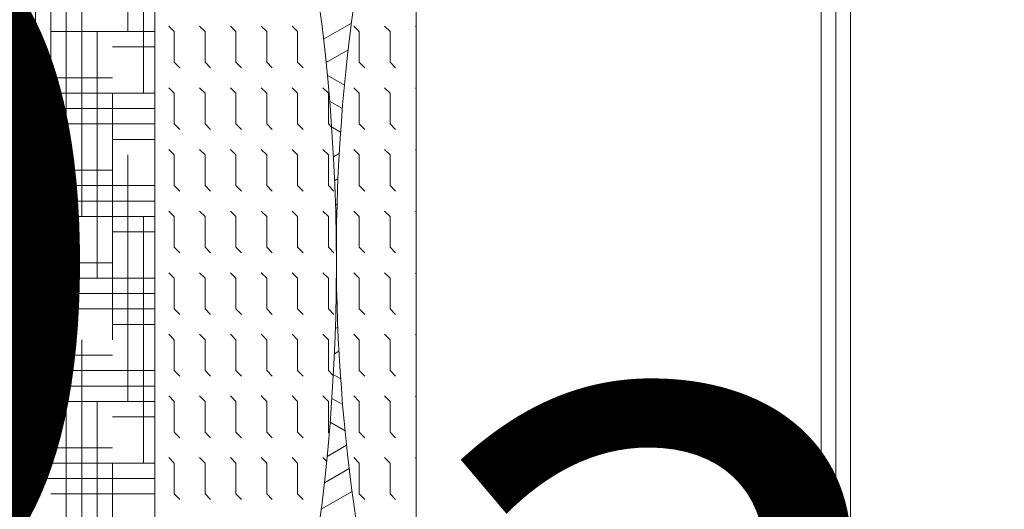
# Model space of a CAD drawing. Units: inches. Extents: x -90 to 536, y -553 to 299.
# Tile 6 of 27: x 96 to 122, y -375 to -362. Entities that reach past the tile are written whole.
import ezdxf

# ---------------------------------------------------------------- set-up
doc = ezdxf.new("R2010")
doc.units = ezdxf.units.IN
doc.layers.add('A-ANNO-DIMS', color=2, linetype='Continuous', lineweight=18)
doc.layers.add('Furniture', color=2, linetype='Continuous', lineweight=18)
doc.styles.get("Standard").update_dxf_attribs({"font": 'arial.ttf'})
doc.dimstyles.get("Standard").update_dxf_attribs({"dimtxt": 18, "dimasz": 12, "dimexe": 0.18, "dimexo": 0.0625, "dimgap": 0.09, "dimtad": 0, "dimtih": 1, "dimtoh": 1, "dimdec": 0, "dimzin": 0, "dimdsep": 46, "dimlunit": 3, "dimtxsty": 'Standard', "dimcen": 0.09, "dimadec": 0, "dimazin": 0, "dimtfac": 1, "dimtdec": 0, "dimtofl": 0, "dimtmove": 0, "dimatfit": 3, "dimfxl": 1, "dimtolj": 1, "dimtzin": 0, "dimarcsym": 0})

# ---------------------------------------------------------------- blocks, each defined once
blk = doc.blocks.new('A$C62731D1C')
for p, q in [((0.10613, 0.66415, 0.68571), (1.46095, 0.66415, 0.68571)), ((0.10613, 0.65215, 0.68571), (1.46095, 0.65215, 0.68571)), ((0.10613, 0.64015, 0.68571), (1.46095, 0.64015, 0.68571)), ((1.39167, 0.31204, 0.68571), (0.17247, 0.31204, 0.68571)), ((0.57908, 0.31135, 0.68571), (0.57977, 0.31204, 0.68571)), ((0.62908, 0.31135, 0.68571), (0.62977, 0.31204, 0.68571)), ((0.67908, 0.31135, 0.68571), (0.67977, 0.31204, 0.68571)), ((0.72908, 0.31135, 0.68571), (0.72977, 0.31204, 0.68571)), ((0.77908, 0.31135, 0.68571), (0.77977, 0.31204, 0.68571)), ((0.82908, 0.31135, 0.68571), (0.82977, 0.31204, 0.68571)), ((0.87908, 0.31135, 0.68571), (0.87977, 0.31204, 0.68571)), ((0.92908, 0.31135, 0.68571), (0.92977, 0.31204, 0.68571)), ((0.57908, 0.28635, 0.68571), (0.5835, 0.29077, 0.68571)), ((0.5835, 0.29077, 0.68571), (0.6085, 0.29077, 0.68571)), ((0.6085, 0.29077, 0.68571), (0.61292, 0.29519, 0.68571)), ((0.62908, 0.28635, 0.68571), (0.6335, 0.29077, 0.68571)), ((0.6335, 0.29077, 0.68571), (0.6585, 0.29077, 0.68571)), ((0.6585, 0.29077, 0.68571), (0.66292, 0.29519, 0.68571)), ((0.67908, 0.28635, 0.68571), (0.6835, 0.29077, 0.68571)), ((0.6835, 0.29077, 0.68571), (0.7085, 0.29077, 0.68571)), ((0.7085, 0.29077, 0.68571), (0.71292, 0.29519, 0.68571)), ((0.72908, 0.28635, 0.68571), (0.7335, 0.29077, 0.68571)), ((0.7335, 0.29077, 0.68571), (0.7585, 0.29077, 0.68571)), ((0.7585, 0.29077, 0.68571), (0.76292, 0.29519, 0.68571)), ((0.77908, 0.28635, 0.68571), (0.7835, 0.29077, 0.68571)), ((0.7835, 0.29077, 0.68571), (0.8085, 0.29077, 0.68571)), ((0.8085, 0.29077, 0.68571), (0.81292, 0.29519, 0.68571)), ((0.82908, 0.28635, 0.68571), (0.8335, 0.29077, 0.68571)), ((0.8335, 0.29077, 0.68571), (0.8585, 0.29077, 0.68571)), ((0.8585, 0.29077, 0.68571), (0.86292, 0.29519, 0.68571)), ((0.87908, 0.28635, 0.68571), (0.8835, 0.29077, 0.68571)), ((0.8835, 0.29077, 0.68571), (0.9085, 0.29077, 0.68571)), ((0.9085, 0.29077, 0.68571), (0.91292, 0.29519, 0.68571)), ((0.92908, 0.28635, 0.68571), (0.9335, 0.29077, 0.68571)), ((0.9335, 0.29077, 0.68571), (0.9585, 0.29077, 0.68571)), ((0.9585, 0.29077, 0.68571), (0.96292, 0.29519, 0.68571)), ((0.57908, 0.26135, 0.68571), (0.5835, 0.26577, 0.68571)), ((0.5835, 0.26577, 0.68571), (0.6085, 0.26577, 0.68571)), ((0.6085, 0.26577, 0.68571), (0.61292, 0.27019, 0.68571)), ((0.62908, 0.26135, 0.68571), (0.6335, 0.26577, 0.68571)), ((0.6335, 0.26577, 0.68571), (0.6585, 0.26577, 0.68571)), ((0.6585, 0.26577, 0.68571), (0.66292, 0.27019, 0.68571)), ((0.67908, 0.26135, 0.68571), (0.6835, 0.26577, 0.68571)), ((0.6835, 0.26577, 0.68571), (0.7085, 0.26577, 0.68571)), ((0.7085, 0.26577, 0.68571), (0.71292, 0.27019, 0.68571)), ((0.72908, 0.26135, 0.68571), (0.7335, 0.26577, 0.68571)), ((0.7335, 0.26577, 0.68571), (0.7585, 0.26577, 0.68571)), ((0.7585, 0.26577, 0.68571), (0.76292, 0.27019, 0.68571)), ((0.77908, 0.26135, 0.68571), (0.7835, 0.26577, 0.68571)), ((0.7835, 0.26577, 0.68571), (0.8085, 0.26577, 0.68571)), ((0.8085, 0.26577, 0.68571), (0.81292, 0.27019, 0.68571)), ((0.82908, 0.26135, 0.68571), (0.8335, 0.26577, 0.68571)), ((0.8335, 0.26577, 0.68571), (0.8585, 0.26577, 0.68571)), ((0.8585, 0.26577, 0.68571), (0.86292, 0.27019, 0.68571)), ((0.87908, 0.26135, 0.68571), (0.8835, 0.26577, 0.68571)), ((0.8835, 0.26577, 0.68571), (0.9085, 0.26577, 0.68571)), ((0.9085, 0.26577, 0.68571), (0.91292, 0.27019, 0.68571)), ((0.92908, 0.26135, 0.68571), (0.9335, 0.26577, 0.68571)), ((0.9335, 0.26577, 0.68571), (0.9585, 0.26577, 0.68571)), ((0.9585, 0.26577, 0.68571), (0.96292, 0.27019, 0.68571)), ((0.57677, 0.25948, 0.68571), (0.58983, 0.23685, 0.68571)), ((0.60866, 0.23889, 0.68571), (0.5983, 0.25682, 0.68571)), ((0.92819, 0.23969, 0.68571), (0.91906, 0.2555, 0.68571)), ((0.93782, 0.25765, 0.68571), (0.94947, 0.23748, 0.68571)), ((0.97092, 0.23496, 0.68571), (0.95645, 0.26002, 0.68571)), ((0.62695, 0.25378, 0.68571), (0.61894, 0.2399, 0.68571)), ((0.64002, 0.24179, 0.68571), (0.64597, 0.25209, 0.68571)), ((0.66513, 0.25064, 0.68571), (0.66094, 0.24338, 0.68571)), ((0.6852, 0.24488, 0.68571), (0.6825, 0.24954, 0.68571)), ((0.70309, 0.24852, 0.68571), (0.70465, 0.24582, 0.68571)), ((0.72425, 0.24652, 0.68571), (0.72351, 0.24779, 0.68571)), ((0.80401, 0.24693, 0.68571), (0.80355, 0.24773, 0.68571)), ((0.82316, 0.2484, 0.68571), (0.82431, 0.24641, 0.68571)), ((0.84477, 0.24562, 0.68571), (0.84263, 0.24932, 0.68571)), ((0.86518, 0.25072, 0.68571), (0.86174, 0.24476, 0.68571)), ((0.88105, 0.24357, 0.68571), (0.88611, 0.25234, 0.68571)), ((0.90723, 0.25428, 0.68571), (0.90024, 0.24216, 0.68571)), ((0.62908, 0.23635, 0.68571), (0.6335, 0.24077, 0.68571)), ((0.6335, 0.24077, 0.68571), (0.6585, 0.24077, 0.68571)), ((0.6585, 0.24077, 0.68571), (0.66112, 0.24339, 0.68571)), ((0.67908, 0.23635, 0.68571), (0.6835, 0.24077, 0.68571)), ((0.6835, 0.24077, 0.68571), (0.7085, 0.24077, 0.68571)), ((0.7085, 0.24077, 0.68571), (0.71292, 0.24519, 0.68571)), ((0.72908, 0.23635, 0.68571), (0.7335, 0.24077, 0.68571)), ((0.7335, 0.24077, 0.68571), (0.7585, 0.24077, 0.68571)), ((0.74324, 0.24737, 0.68571), (0.74302, 0.24697, 0.68571)), ((0.7585, 0.24077, 0.68571), (0.76292, 0.24519, 0.68571)), ((0.77908, 0.23635, 0.68571), (0.7835, 0.24077, 0.68571)), ((0.78322, 0.24733, 0.68571), (0.78315, 0.24721, 0.68571)), ((0.7835, 0.24077, 0.68571), (0.8085, 0.24077, 0.68571)), ((0.8085, 0.24077, 0.68571), (0.81292, 0.24519, 0.68571)), ((0.82908, 0.23635, 0.68571), (0.8335, 0.24077, 0.68571)), ((0.8335, 0.24077, 0.68571), (0.8585, 0.24077, 0.68571)), ((0.8585, 0.24077, 0.68571), (0.86246, 0.24472, 0.68571)), ((0.87908, 0.23635, 0.68571), (0.8835, 0.24077, 0.68571)), ((0.8835, 0.24077, 0.68571), (0.9085, 0.24077, 0.68571)), ((0.9085, 0.24077, 0.68571), (0.90916, 0.24143, 0.68571)), ((0.92908, 0.23635, 0.68571), (0.93204, 0.23931, 0.68571)), ((0.57908, 0.21135, 0.68571), (0.5835, 0.21577, 0.68571)), ((0.5835, 0.21577, 0.68571), (0.6085, 0.21577, 0.68571)), ((0.6085, 0.21577, 0.68571), (0.61292, 0.22019, 0.68571)), ((0.62908, 0.21135, 0.68571), (0.6335, 0.21577, 0.68571)), ((0.6335, 0.21577, 0.68571), (0.6585, 0.21577, 0.68571)), ((0.6585, 0.21577, 0.68571), (0.66292, 0.22019, 0.68571)), ((0.67908, 0.21135, 0.68571), (0.6835, 0.21577, 0.68571)), ((0.6835, 0.21577, 0.68571), (0.7085, 0.21577, 0.68571)), ((0.7085, 0.21577, 0.68571), (0.71292, 0.22019, 0.68571)), ((0.72908, 0.21135, 0.68571), (0.7335, 0.21577, 0.68571)), ((0.7335, 0.21577, 0.68571), (0.7585, 0.21577, 0.68571)), ((0.7585, 0.21577, 0.68571), (0.76292, 0.22019, 0.68571)), ((0.77908, 0.21135, 0.68571), (0.7835, 0.21577, 0.68571)), ((0.7835, 0.21577, 0.68571), (0.8085, 0.21577, 0.68571)), ((0.8085, 0.21577, 0.68571), (0.81292, 0.22019, 0.68571)), ((0.82908, 0.21135, 0.68571), (0.8335, 0.21577, 0.68571)), ((0.8335, 0.21577, 0.68571), (0.8585, 0.21577, 0.68571)), ((0.8585, 0.21577, 0.68571), (0.86292, 0.22019, 0.68571)), ((0.87908, 0.21135, 0.68571), (0.8835, 0.21577, 0.68571)), ((0.8835, 0.21577, 0.68571), (0.9085, 0.21577, 0.68571)), ((0.9085, 0.21577, 0.68571), (0.91292, 0.22019, 0.68571)), ((0.92908, 0.21135, 0.68571), (0.9335, 0.21577, 0.68571)), ((0.9335, 0.21577, 0.68571), (0.9585, 0.21577, 0.68571)), ((0.9585, 0.21577, 0.68571), (0.96292, 0.22019, 0.68571)), ((0.6085, 0.19077, 0.68571), (0.61292, 0.19519, 0.68571)), ((0.6585, 0.19077, 0.68571), (0.66292, 0.19519, 0.68571)), ((0.7085, 0.19077, 0.68571), (0.71292, 0.19519, 0.68571)), ((0.7585, 0.19077, 0.68571), (0.76292, 0.19519, 0.68571)), ((0.8085, 0.19077, 0.68571), (0.81292, 0.19519, 0.68571)), ((0.8585, 0.19077, 0.68571), (0.86292, 0.19519, 0.68571)), ((0.9085, 0.19077, 0.68571), (0.91292, 0.19519, 0.68571)), ((0.9585, 0.19077, 0.68571), (0.96292, 0.19519, 0.68571)), ((0.57908, 0.18635, 0.68571), (0.5835, 0.19077, 0.68571)), ((0.5835, 0.19077, 0.68571), (0.6085, 0.19077, 0.68571)), ((0.62908, 0.18635, 0.68571), (0.6335, 0.19077, 0.68571)), ((0.6335, 0.19077, 0.68571), (0.6585, 0.19077, 0.68571)), ((0.67908, 0.18635, 0.68571), (0.6835, 0.19077, 0.68571)), ((0.6835, 0.19077, 0.68571), (0.7085, 0.19077, 0.68571)), ((0.72908, 0.18635, 0.68571), (0.7335, 0.19077, 0.68571)), ((0.7335, 0.19077, 0.68571), (0.7585, 0.19077, 0.68571)), ((0.77908, 0.18635, 0.68571), (0.7835, 0.19077, 0.68571)), ((0.7835, 0.19077, 0.68571), (0.8085, 0.19077, 0.68571)), ((0.82908, 0.18635, 0.68571), (0.8335, 0.19077, 0.68571)), ((0.8335, 0.19077, 0.68571), (0.8585, 0.19077, 0.68571)), ((0.87908, 0.18635, 0.68571), (0.8835, 0.19077, 0.68571)), ((0.8835, 0.19077, 0.68571), (0.9085, 0.19077, 0.68571)), ((0.92908, 0.18635, 0.68571), (0.9335, 0.19077, 0.68571)), ((0.9335, 0.19077, 0.68571), (0.9585, 0.19077, 0.68571)), ((0.6085, 0.16577, 0.68571), (0.61292, 0.17019, 0.68571)), ((0.6585, 0.16577, 0.68571), (0.66292, 0.17019, 0.68571)), ((0.7085, 0.16577, 0.68571), (0.71292, 0.17019, 0.68571)), ((0.7585, 0.16577, 0.68571), (0.76292, 0.17019, 0.68571)), ((0.8085, 0.16577, 0.68571), (0.81292, 0.17019, 0.68571)), ((0.8585, 0.16577, 0.68571), (0.86292, 0.17019, 0.68571)), ((0.9085, 0.16577, 0.68571), (0.91292, 0.17019, 0.68571)), ((0.9585, 0.16577, 0.68571), (0.96292, 0.17019, 0.68571)), ((0.57908, 0.16135, 0.68571), (0.5835, 0.16577, 0.68571)), ((0.5835, 0.16577, 0.68571), (0.6085, 0.16577, 0.68571)), ((0.62908, 0.16135, 0.68571), (0.6335, 0.16577, 0.68571)), ((0.6335, 0.16577, 0.68571), (0.6585, 0.16577, 0.68571)), ((0.67908, 0.16135, 0.68571), (0.6835, 0.16577, 0.68571)), ((0.6835, 0.16577, 0.68571), (0.7085, 0.16577, 0.68571)), ((0.72908, 0.16135, 0.68571), (0.7335, 0.16577, 0.68571)), ((0.7335, 0.16577, 0.68571), (0.7585, 0.16577, 0.68571)), ((0.77908, 0.16135, 0.68571), (0.7835, 0.16577, 0.68571)), ((0.7835, 0.16577, 0.68571), (0.8085, 0.16577, 0.68571)), ((0.82908, 0.16135, 0.68571), (0.8335, 0.16577, 0.68571)), ((0.8335, 0.16577, 0.68571), (0.8585, 0.16577, 0.68571)), ((0.87908, 0.16135, 0.68571), (0.8835, 0.16577, 0.68571)), ((0.8835, 0.16577, 0.68571), (0.9085, 0.16577, 0.68571)), ((0.92908, 0.16135, 0.68571), (0.9335, 0.16577, 0.68571)), ((0.9335, 0.16577, 0.68571), (0.9585, 0.16577, 0.68571)), ((0.6085, 0.14077, 0.68571), (0.61292, 0.14519, 0.68571)), ((0.6585, 0.14077, 0.68571), (0.66292, 0.14519, 0.68571)), ((0.7085, 0.14077, 0.68571), (0.71292, 0.14519, 0.68571)), ((0.7585, 0.14077, 0.68571), (0.76292, 0.14519, 0.68571)), ((0.8085, 0.14077, 0.68571), (0.81292, 0.14519, 0.68571)), ((0.8585, 0.14077, 0.68571), (0.86292, 0.14519, 0.68571)), ((0.9085, 0.14077, 0.68571), (0.91292, 0.14519, 0.68571)), ((0.9585, 0.14077, 0.68571), (0.96292, 0.14519, 0.68571)), ((0.57908, 0.13635, 0.68571), (0.5835, 0.14077, 0.68571)), ((0.5835, 0.14077, 0.68571), (0.6085, 0.14077, 0.68571)), ((0.62908, 0.13635, 0.68571), (0.6335, 0.14077, 0.68571)), ((0.6335, 0.14077, 0.68571), (0.6585, 0.14077, 0.68571)), ((0.67908, 0.13635, 0.68571), (0.6835, 0.14077, 0.68571)), ((0.6835, 0.14077, 0.68571), (0.7085, 0.14077, 0.68571)), ((0.72908, 0.13635, 0.68571), (0.7335, 0.14077, 0.68571)), ((0.7335, 0.14077, 0.68571), (0.7585, 0.14077, 0.68571)), ((0.77908, 0.13635, 0.68571), (0.7835, 0.14077, 0.68571)), ((0.7835, 0.14077, 0.68571), (0.8085, 0.14077, 0.68571)), ((0.82908, 0.13635, 0.68571), (0.8335, 0.14077, 0.68571)), ((0.8335, 0.14077, 0.68571), (0.8585, 0.14077, 0.68571)), ((0.87908, 0.13635, 0.68571), (0.8835, 0.14077, 0.68571)), ((0.8835, 0.14077, 0.68571), (0.9085, 0.14077, 0.68571)), ((0.92908, 0.13635, 0.68571), (0.9335, 0.14077, 0.68571)), ((0.9335, 0.14077, 0.68571), (0.9585, 0.14077, 0.68571)), ((0.6085, 0.11577, 0.68571), (0.61292, 0.12019, 0.68571)), ((0.6585, 0.11577, 0.68571), (0.66292, 0.12019, 0.68571)), ((0.7085, 0.11577, 0.68571), (0.71292, 0.12019, 0.68571)), ((0.7585, 0.11577, 0.68571), (0.76292, 0.12019, 0.68571)), ((0.8085, 0.11577, 0.68571), (0.81292, 0.12019, 0.68571)), ((0.8585, 0.11577, 0.68571), (0.86292, 0.12019, 0.68571)), ((0.9085, 0.11577, 0.68571), (0.91292, 0.12019, 0.68571)), ((0.9585, 0.11577, 0.68571), (0.96292, 0.12019, 0.68571)), ((0.57908, 0.11135, 0.68571), (0.5835, 0.11577, 0.68571)), ((0.5835, 0.11577, 0.68571), (0.6085, 0.11577, 0.68571)), ((0.62908, 0.11135, 0.68571), (0.6335, 0.11577, 0.68571)), ((0.6335, 0.11577, 0.68571), (0.6585, 0.11577, 0.68571)), ((0.67908, 0.11135, 0.68571), (0.6835, 0.11577, 0.68571)), ((0.6835, 0.11577, 0.68571), (0.7085, 0.11577, 0.68571)), ((0.72908, 0.11135, 0.68571), (0.7335, 0.11577, 0.68571)), ((0.7335, 0.11577, 0.68571), (0.7585, 0.11577, 0.68571)), ((0.77908, 0.11135, 0.68571), (0.7835, 0.11577, 0.68571)), ((0.7835, 0.11577, 0.68571), (0.8085, 0.11577, 0.68571)), ((0.82908, 0.11135, 0.68571), (0.8335, 0.11577, 0.68571)), ((0.8335, 0.11577, 0.68571), (0.8585, 0.11577, 0.68571)), ((0.87908, 0.11135, 0.68571), (0.8835, 0.11577, 0.68571)), ((0.8835, 0.11577, 0.68571), (0.9085, 0.11577, 0.68571)), ((0.92908, 0.11135, 0.68571), (0.9335, 0.11577, 0.68571)), ((0.9335, 0.11577, 0.68571), (0.9585, 0.11577, 0.68571)), ((1.44488, 0.1, 0.68571), (0.1, 0.1, 0.68571)), ((0.5835, 0.01577, 0.68571), (0.5835, 0.1, 0.68571)), ((0.596, 0.06577, 0.68571), (0.596, 0.1, 0.68571)), ((0.6335, 0, 0.68571), (0.6335, 0.1, 0.68571)), ((0.646, 0, 0.68571), (0.646, 0.1, 0.68571)), ((0.6585, 0.01577, 0.68571), (0.6585, 0.1, 0.68571)), ((0.671, 0.06577, 0.68571), (0.671, 0.1, 0.68571)), ((0.7085, 0, 0.68571), (0.7085, 0.1, 0.68571)), ((0.721, 0, 0.68571), (0.721, 0.1, 0.68571)), ((0.7335, 0.01577, 0.68571), (0.7335, 0.1, 0.68571)), ((0.746, 0.06577, 0.68571), (0.746, 0.1, 0.68571)), ((0.7835, 0, 0.68571), (0.7835, 0.1, 0.68571)), ((0.796, 0, 0.68571), (0.796, 0.1, 0.68571)), ((0.8085, 0.01577, 0.68571), (0.8085, 0.1, 0.68571)), ((0.821, 0.06577, 0.68571), (0.821, 0.1, 0.68571)), ((0.8585, 0, 0.68571), (0.8585, 0.1, 0.68571)), ((0.871, 0, 0.68571), (0.871, 0.1, 0.68571)), ((0.8835, 0.01577, 0.68571), (0.8835, 0.1, 0.68571)), ((0.896, 0.06577, 0.68571), (0.896, 0.1, 0.68571)), ((0.9335, 0, 0.68571), (0.9335, 0.1, 0.68571)), ((0.946, 0, 0.68571), (0.946, 0.1, 0.68571)), ((0.9585, 0.01577, 0.68571), (0.9585, 0.1, 0.68571)), ((0.4335, 0.09077, 0.68571), (0.6335, 0.09077, 0.68571)), ((0.7335, 0.09077, 0.68571), (0.9335, 0.09077, 0.68571)), ((0.3835, 0.07827, 0.68571), (0.5835, 0.07827, 0.68571)), ((0.6835, 0.07827, 0.68571), (0.8835, 0.07827, 0.68571)), ((0.621, 0, 0.68571), (0.621, 0.06577, 0.68571)), ((0.6335, 0.06577, 0.68571), (0.8335, 0.06577, 0.68571)), ((0.696, 0, 0.68571), (0.696, 0.06577, 0.68571)), ((0.771, 0, 0.68571), (0.771, 0.06577, 0.68571)), ((0.846, 0, 0.68571), (0.846, 0.06577, 0.68571)), ((0.921, 0, 0.68571), (0.921, 0.06577, 0.68571)), ((0.9335, 0.06577, 0.68571), (1.1335, 0.06577, 0.68571)), ((0.5835, 0.05327, 0.68571), (0.7835, 0.05327, 0.68571)), ((0.8835, 0.05327, 0.68571), (1.0835, 0.05327, 0.68571)), ((0.5335, 0.04077, 0.68571), (0.7335, 0.04077, 0.68571)), ((0.8335, 0.04077, 0.68571), (1.0335, 0.04077, 0.68571)), ((0.4835, 0.02827, 0.68571), (0.6835, 0.02827, 0.68571)), ((0.7835, 0.02827, 0.68571), (0.9835, 0.02827, 0.68571)), ((0.4335, 0.01577, 0.68571), (0.6335, 0.01577, 0.68571)), ((0.6085, 0, 0.68571), (0.6085, 0.01577, 0.68571)), ((0.6835, 0, 0.68571), (0.6835, 0.01577, 0.68571)), ((0.7335, 0.01577, 0.68571), (0.9335, 0.01577, 0.68571)), ((0.7585, 0, 0.68571), (0.7585, 0.01577, 0.68571)), ((0.8335, 0, 0.68571), (0.8335, 0.01577, 0.68571)), ((0.9085, 0, 0.68571), (0.9085, 0.01577, 0.68571)), ((0.3835, 0.00327, 0.68571), (0.5835, 0.00327, 0.68571)), ((0.6835, 0.00327, 0.68571), (0.8835, 0.00327, 0.68571))]:
    blk.add_line(p, q)
for centre, radius, start, end in [((0.76456, 1.69033, 0.68571), 1.44313, 252.76056, 287.23944), ((0.77244, -1.36185, 0.68571), 1.6091, 65.29791, 114.70209)]:
    blk.add_arc(centre, radius, start, end)
blk = doc.blocks.new('A$C0E6D7E3D')
blk.add_blockref('A$C62731D1C', (0, 0))
blk = doc.blocks.new('*D28')
at = {"layer": 'A-ANNO-DIMS', "color": 0, "lineweight": -2, "transparency": 16777216}
for p, q in [((92.257, -392.554), (92.257, -380.554)), ((92.257, -380.554), (104.257, -380.554)), ((86.694, -392.554), (92.437, -392.554)), ((92.257, -416.554), (92.257, -404.554)), ((86.694, -428.554), (92.437, -428.554))]:
    blk.add_line(p, q, dxfattribs=at)
at = {"layer": 'A-ANNO-DIMS', "color": 0, "transparency": 16777216}
for points in [[(90.257, -404.554), (94.257, -404.554), (92.257, -392.554)], [(90.257, -416.554), (94.257, -416.554), (92.257, -428.554)]]:
    blk.add_solid(points, dxfattribs=at)
at = {"layer": 'Defpoints', "color": 0, "transparency": 16777216}
for p in [(86.632, -392.554), (92.257, -392.554), (86.632, -428.554)]:
    blk.add_point(p, dxfattribs=at)
at = {"layer": 'A-ANNO-DIMS', "color": 0, "transparency": 16777216, "insert": (148.15, -380.554), "char_height": 18, "attachment_point": 5}
blk.add_mtext('\\A1;36 TYP.', dxfattribs=at)
blk = doc.blocks.new('*D46')
at = {"layer": 'A-ANNO-DIMS', "color": 0, "lineweight": -2, "transparency": 16777216}
for p, q in [((92.796, -304.194), (92.796, -292.194)), ((96.856, -316.194), (92.616, -316.194)), ((96.856, -332.226), (92.616, -332.226)), ((92.796, -344.226), (92.796, -356.226)), ((92.796, -356.226), (80.796, -356.226))]:
    blk.add_line(p, q, dxfattribs=at)
at = {"layer": 'A-ANNO-DIMS', "color": 0, "transparency": 16777216}
for points in [[(90.796, -304.194), (94.796, -304.194), (92.796, -316.194)], [(90.796, -344.226), (94.796, -344.226), (92.796, -332.226)]]:
    blk.add_solid(points, dxfattribs=at)
at = {"layer": 'Defpoints', "color": 0, "transparency": 16777216}
for p in [(96.919, -316.194), (92.796, -332.226), (96.919, -332.226)]:
    blk.add_point(p, dxfattribs=at)
at = {"layer": 'A-ANNO-DIMS', "color": 0, "transparency": 16777216, "insert": (68.667, -356.226), "char_height": 18, "attachment_point": 5}
blk.add_mtext('\\A1;16', dxfattribs=at)
blk = doc.blocks.new('*D51')
at = {"layer": 'A-ANNO-DIMS', "color": 0, "lineweight": -2, "transparency": 16777216}
for p, q in [((96.806, -393.34), (96.806, -404.606)), ((171.132, -393.34), (171.132, -404.606)), ((108.806, -404.426), (159.132, -404.426)), ((171.132, -404.426), (183.132, -404.426))]:
    blk.add_line(p, q, dxfattribs=at)
at = {"layer": 'A-ANNO-DIMS', "color": 0, "transparency": 16777216}
for points in [[(108.806, -402.426), (108.806, -406.426), (96.806, -404.426)], [(159.132, -402.426), (159.132, -406.426), (171.132, -404.426)]]:
    blk.add_solid(points, dxfattribs=at)
at = {"layer": 'Defpoints', "color": 0, "transparency": 16777216}
for p in [(96.806, -393.277), (171.132, -393.277), (171.132, -404.426)]:
    blk.add_point(p, dxfattribs=at)
at = {"layer": 'A-ANNO-DIMS', "color": 0, "transparency": 16777216, "insert": (274.99, -404.426), "char_height": 18, "attachment_point": 5}
blk.add_mtext('\\A1;SINGLE BED 74', dxfattribs=at)
blk = doc.blocks.new('*D52')
at = {"layer": 'A-ANNO-DIMS', "color": 0, "lineweight": -2, "transparency": 16777216}
for p, q in [((96.743, -343.206), (85.477, -343.206)), ((85.657, -355.206), (85.657, -358.961)), ((85.657, -381.277), (85.657, -377.522)), ((96.743, -393.277), (85.477, -393.277))]:
    blk.add_line(p, q, dxfattribs=at)
at = {"layer": 'A-ANNO-DIMS', "color": 0, "transparency": 16777216}
for points in [[(83.657, -355.206), (87.657, -355.206), (85.657, -343.206)], [(83.657, -381.277), (87.657, -381.277), (85.657, -393.277)]]:
    blk.add_solid(points, dxfattribs=at)
at = {"layer": 'Defpoints', "color": 0, "transparency": 16777216}
for p in [(96.806, -343.206), (85.657, -393.277), (96.806, -393.277)]:
    blk.add_point(p, dxfattribs=at)
at = {"layer": 'A-ANNO-DIMS', "color": 0, "transparency": 16777216, "insert": (85.657, -368.242), "char_height": 18, "attachment_point": 5}
blk.add_mtext('\\A1;50', dxfattribs=at)
blk = doc.blocks.new('*D54')
at = {"layer": 'A-ANNO-DIMS', "color": 0, "lineweight": -2, "transparency": 16777216}
for p, q in [((113.069, 249.446), (-2.848, 249.446)), ((-2.668, 237.446), (-2.668, -117.767)), ((-2.668, -491.554), (-2.668, -136.34)), ((38.069, -503.554), (-2.848, -503.554))]:
    blk.add_line(p, q, dxfattribs=at)
at = {"layer": 'A-ANNO-DIMS', "color": 0, "transparency": 16777216}
for points in [[(-4.668, 237.446), (-0.668, 237.446), (-2.668, 249.446)], [(-4.668, -491.554), (-0.668, -491.554), (-2.668, -503.554)]]:
    blk.add_solid(points, dxfattribs=at)
at = {"layer": 'Defpoints', "color": 0, "transparency": 16777216}
for p in [(-2.668, 249.446), (113.132, 249.446), (38.132, -503.554)]:
    blk.add_point(p, dxfattribs=at)
at = {"layer": 'A-ANNO-DIMS', "color": 0, "transparency": 16777216, "insert": (-2.668, -127.054), "char_height": 18, "attachment_point": 5}
blk.add_mtext('\\A1;753', dxfattribs=at)

msp = doc.modelspace()

# ---------------------------------------------------------------- block references
at = {"layer": 'Furniture', "xscale": 32.41097235378273, "yscale": 32.41097235378273, "zscale": 32.41097235378273, "rotation": 270}
msp.add_blockref('A$C0E6D7E3D', (96.8056, -343.2061, -22.2246), dxfattribs=at)

# ---------------------------------------------------------------- dimensions: what is measured, and where the dimension line sits
at = {"layer": 'A-ANNO-DIMS'}
for base, p1, p2, angle, picture, middle in [((-2.6677, 249.4462), (38.1317, -503.5538), (113.1317, 249.4462), 90, '*D54', (-2.6677, -127.0538)), ((92.7963, -332.2258), (96.9187, -316.194), (96.9187, -332.2258), 270, '*D46', (68.6674, -356.2258)), ((85.6567, -393.2773), (96.8056, -343.2061), (96.8056, -393.2773), 270, '*D52', (85.6567, -368.2417))]:
    dim = msp.add_linear_dim(base=base, p1=p1, p2=p2, angle=angle, dimstyle='Standard', override={"dimdec": 0, "dimlfac": 1, "dimrnd": 0, "dimzin": 0, "dimdsep": 46, "dimlunit": 2}, dxfattribs=at)
    dim.commit()
    dim.dimension.update_dxf_attribs({"geometry": picture, "text_midpoint": middle})
dim = msp.add_linear_dim(base=(92.2567, -392.5538), p1=(86.6317, -428.5538), p2=(86.6317, -392.5538), angle=90, text='<> TYP.', dimstyle='Standard', override={"dimdec": 0, "dimlfac": 1, "dimrnd": 0, "dimzin": 0, "dimdsep": 46, "dimlunit": 2}, dxfattribs=at)
dim.commit()
dim.dimension.update_dxf_attribs({"geometry": '*D28', "text_midpoint": (148.1496, -380.5538)})
dim = msp.add_linear_dim(base=(171.1317, -404.4263), p1=(96.8056, -393.2773), p2=(171.1317, -393.2773), text='SINGLE BED <>', dimstyle='Standard', override={"dimdec": 0, "dimlfac": 1, "dimrnd": 0, "dimzin": 0, "dimdsep": 46, "dimlunit": 2}, dxfattribs=at)
dim.commit()
dim.dimension.update_dxf_attribs({"geometry": '*D51', "text_midpoint": (274.9898, -404.4263)})

doc.saveas('drawing.dxf')
